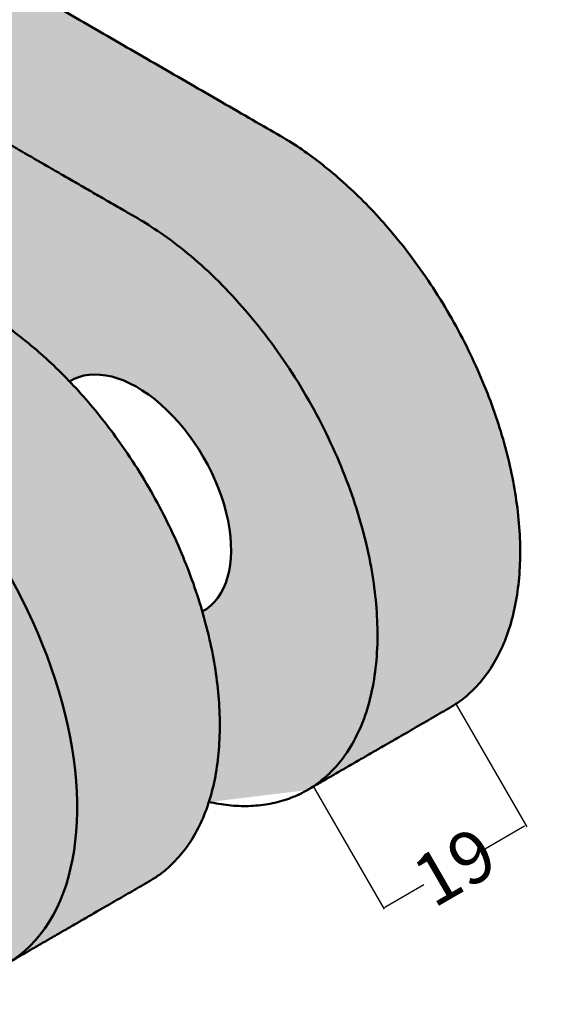
# Model space of a CAD drawing. Units: millimetres. Extents: x -24 to 183, y 0 to 191.
# Tile 1 of 1: x 120.7 to 183.4, y 6.1 to 119.6. Entities that reach past the tile are written whole.
import ezdxf

# ---------------------------------------------------------------- set-up
doc = ezdxf.new("R2010")
doc.units = ezdxf.units.MM
doc.header["$MEASUREMENT"] = 0
for name, color, linetype, lineweight in [('M-DIMS', 2, 'Continuous', 25), ('M-HATC', 7, 'Continuous', 18), ('M-OUTL', 7, 'Continuous', 50)]:
    doc.layers.add(name, color=color, linetype=linetype, lineweight=lineweight)
doc.styles.get("Standard").update_dxf_attribs({"font": 'arial.ttf'})
doc.dimstyles.get("Standard").update_dxf_attribs({"dimtxt": 6, "dimasz": 0.18, "dimexe": 0.18, "dimexo": 0.0625, "dimgap": 0.09, "dimtad": 0, "dimtoh": 1, "dimdec": 0, "dimzin": 0, "dimdsep": 46, "dimtxsty": 'Standard', "dimcen": 0.09, "dimadec": 0, "dimazin": 0, "dimtfac": 1, "dimtdec": 0, "dimtofl": 0, "dimtmove": 0, "dimatfit": 3, "dimfxl": 1, "dimtolj": 1, "dimtzin": 0, "dimarcsym": 0})

# ---------------------------------------------------------------- blocks, each defined once
blk = doc.blocks.new('*D10')
at = {"layer": 'Defpoints', "color": 0, "transparency": 16777216}
for p in [(171.0477061015821, 40.70913944972441), (154.5932234296778, 31.20913944972442), (179.1326412495718, 26.70562099750689)]:
    blk.add_point(p, dxfattribs=at)
at = {"layer": 'M-DIMS', "color": 0, "lineweight": -2, "transparency": 16777216}
for p, q in [((171.0789561015821, 40.65501286198788), (179.2226412495718, 26.54973642482568)), ((154.6244734296777, 31.15501286198789), (162.7681585776674, 17.04973642482568)), ((178.9767566768906, 26.61562099750689), (174.4657567670197, 24.01119398522857)), ((162.8340431503486, 17.29562099750689), (167.3450430602194, 19.90004800978519))]:
    blk.add_line(p, q, dxfattribs=at)
at = {"layer": 'M-DIMS', "color": 0, "transparency": 16777216}
for points in [[(178.9617566768906, 26.64160175962042), (178.9917566768906, 26.58964023539335), (179.1326412495718, 26.70562099750689)], [(162.8190431503487, 17.32160175962043), (162.8490431503486, 17.26964023539335), (162.6781585776674, 17.20562099750689)]]:
    blk.add_solid(points, dxfattribs=at)
at = {"layer": 'M-DIMS', "color": 0, "transparency": 16777216, "insert": (170.9053999136196, 21.95562099750688), "char_height": 6, "attachment_point": 5, "rotation": 29.999999999999993}
blk.add_mtext('\\A1;19', dxfattribs=at)

msp = doc.modelspace()

# ---------------------------------------------------------------- hatches: boundary and pattern name
at = {"layer": 'M-HATC'}
h = msp.add_hatch(color=256, dxfattribs=at)
h.set_gradient(color1=(244, 238, 81), color2=(244, 238, 81), tint=1)
h.paths.add_polyline_path([(64.14245464474502, 175.211638219327), (-0.8094506390879131, 137.7116382193271), (53.75014979933173, 106.2116382193271), (118.7020550831646, 143.7116382193271)])
edge = h.paths.add_edge_path()
edge.add_line((95.31936918098478, 130.2116382193271), (77.13283570151161, 119.7116382193271))
edge.add_spline(control_points=[(77.13283570151158, 119.7116382193271), (89.17924906810929, 107.2566382193724), (101.2256624347508, 94.80163821937239)], knot_values=[5.356194490192345, 5.356194490192345, 5.356194490192345, 6.356194490188707, 6.356194490192345, 6.356194490192345], weights=[1, 1, 1], degree=2, periodic=0)
edge.add_spline(control_points=[(101.2256624347947, 94.80163821932707), (110.3189291745312, 100.051638219327), (119.4121959142679, 105.301638219327)], knot_values=[6.356194490188707, 6.356194490192345, 6.356194490192345, 7.356194490192345, 7.356194490192345, 7.356194490192345], weights=[1, 1, 1], degree=2, periodic=0)
edge.add_line((119.4121959142679, 105.3016382193271), (95.31936918098478, 130.2116382193271))
edge = h.paths.add_edge_path()
edge.add_spline(control_points=[(150.7449950231889, 106.2116382193271), (134.7235250531767, 115.4616382193271), (118.7020550831646, 124.7116382193271)], knot_values=[3.356194490192345, 3.356194490192345, 3.356194490192345, 4.178416712414569, 4.178416712414569, 4.178416712414569], weights=[1, 1, 1], degree=2, periodic=0)
edge.add_spline(control_points=[(118.7020550831646, 124.7116382193271), (115.2379534680269, 126.7116382193271), (111.7738518528891, 128.7116382193271)], knot_values=[4.178416712414569, 4.178416712414569, 4.178416712414569, 4.356194490192345, 4.356194490192345, 4.356194490192345], weights=[1, 1, 1], degree=2, periodic=0)
edge.add_spline(control_points=[(111.7738518528891, 128.7116382193271), (106.960071285434, 125.9324007128871), (102.1462907179789, 123.1531632064471)], knot_values=[4.356194490192345, 4.356194490192345, 4.356194490192345, 5.356194490192345, 5.356194490192345, 5.356194490192345], weights=[1, 1, 1], degree=2, periodic=0)
edge.add_line((102.1462907179789, 123.1531632064471), (119.4121959142679, 105.301638219327))
edge.add_spline(control_points=[(119.4121959142679, 105.301638219327), (126.8513541327762, 101.006638219327), (134.2905123512845, 96.71163821932709)], knot_values=[7.356194490192345, 7.356194490192345, 7.356194490192345, 8.356194490192346, 8.356194490192346, 8.356194490192346], weights=[1, 1, 1], degree=2, periodic=0)
edge.add_spline(control_points=[(134.2905123512845, 96.71163821932709), (158.0953395036126, 82.96791485491796), (161.6862132372617, 53.72180942535438), (165.2770869709107, 24.47570399579081), (142.5556009483879, 29.39608484008592)], knot_values=[8.356194490192346, 8.356194490192346, 8.356194490192346, 9.775566349411587, 9.775566349411587, 11.19493820863083, 11.19493820863083, 11.19493820863083], weights=[1, 0.7585665602715825, 1, 0.7585665602715825, 1], degree=2, periodic=0)
edge.add_spline(control_points=[(153.8864302935499, 30.77051272237281), (162.1136716295021, 35.52051272237281), (170.3409129654543, 40.2705127223728)], knot_values=[0, 0, 0, 1, 1, 1], weights=[1, 1, 1], degree=2, periodic=0)
edge.add_spline(control_points=[(170.3409129654543, 40.2705127223728), (183.4344867248955, 47.83009105704043), (176.3482956693094, 71.67543553482938), (169.2621046137232, 95.5207800126183), (150.7449950231889, 106.2116382193271)], knot_values=[1, 1, 1, 2.178097245096171, 2.178097245096171, 3.356194490192345, 3.356194490192345, 3.356194490192345], weights=[1, 0.831469612302545, 1, 0.831469612302545, 1], degree=2, periodic=0)
edge = h.paths.add_edge_path(flags=17)
edge.add_spline(control_points=[(134.2905123512845, 96.71163821932709), (126.8513541327762, 101.006638219327), (119.4121959142679, 105.301638219327)], knot_values=[7.356194490192345, 7.356194490192345, 7.356194490192345, 8.356194490192346, 8.356194490192346, 8.356194490192346], weights=[1, 1, 1], degree=2, periodic=0)
edge.add_line((119.4121959142679, 105.301638219327), (119.4121959142679, 84.07281383496964))
edge.add_spline(control_points=[(119.4121959142679, 84.07281383496964), (123.0724490086632, 81.4513939238958), (126.4903518736498, 77.88262675949477)], knot_values=[2.966768687208849, 2.966768687208849, 2.966768687208849, 3.231438789490306, 3.231438789490306, 3.231438789490306], weights=[0.9680864183363699, 0.938243390584542, 0.9254123758008628], degree=2, periodic=0)
edge.add_ellipse((134.2905123512845, 64.71163821932709), major_axis=(7.654655446197426, -13.25825214724777), ratio=0.5773502691896262, start_angle=359.3650130620468, end_angle=540.634986937953, ccw=False)
edge.add_spline(control_points=[(141.7968427812057, 51.37100682201758), (145.5119247027769, 38.61436904653682), (142.5556009483879, 29.39608484008592)], knot_values=[1.485548755374229, 1.485548755374229, 1.485548755374229, 2.169061485720957, 2.169061485720957, 2.169061485720957], weights=[0.9974346422091759, 0.9011559533067647, 0.9183363162707197], degree=2, periodic=0)
edge.add_spline(control_points=[(142.5556009483879, 29.39608484008592), (165.2770869709107, 24.47570399579081), (161.6862132372617, 53.72180942535438), (158.0953395036126, 82.96791485491796), (134.2905123512845, 96.71163821932709)], knot_values=[8.356194490192342, 8.356194490192342, 8.356194490192342, 9.775566349411587, 9.775566349411587, 11.19493820863083, 11.19493820863083, 11.19493820863083], weights=[1, 0.7585665602715825, 1, 0.7585665602715825, 1], degree=2, periodic=0)
edge = h.paths.add_edge_path()
edge.add_spline(control_points=[(119.4121959142679, 105.301638219327), (110.3189291745312, 100.051638219327), (101.2256624347947, 94.80163821932707)], knot_values=[6.356194490188707, 6.356194490188707, 6.356194490188707, 7.356194490188707, 7.356194490188707, 7.356194490192345], weights=[1, 1, 1], degree=2, periodic=0)
edge.add_spline(control_points=[(101.2256624347947, 94.80163821932709), (108.664820653303, 90.5066382193271), (116.1039788718113, 86.21163821932711)], knot_values=[3.356194490192346, 3.356194490192346, 3.356194490192346, 3.737972267970123, 3.737972267970123, 3.737972267970123], weights=[1, 1, 1], degree=2, periodic=0)
edge.add_spline(control_points=[(116.1039788718113, 86.21163821932711), (117.7640226821475, 85.25321147856292), (119.4121959142679, 84.07281383496964)], knot_values=[3.231438789490306, 3.231438789490306, 3.231438789490306, 3.356194490192346, 3.356194490192346, 3.356194490192346], weights=[1, 0.9821533182474542, 0.9680864183363699], degree=2, periodic=0)
edge.add_line((119.4121959142679, 84.07281383496965), (119.4121959142679, 105.301638219327))
h.paths.add_polyline_path([(-0.8094506390879131, 137.7116382193271), (-0.8094506390879131, 117.7116382193271), (32.09951470472076, 98.71163821932709), (32.09951470472076, 63.71163821932707), (-0.8094506390879131, 82.71163821932709), (-0.8094506390879062, 62.71163821932709), (53.75014979933173, 31.21163821932709), (53.75014979933173, 106.2116382193271)])
h.paths.add_polyline_path([(32.09951470472076, 98.71163821932709), (29.50143849336745, 100.2116382193271), (-0.8094506390879203, 82.71163821932709), (32.09951470472076, 63.71163821932708)])
edge = h.paths.add_edge_path()
edge.add_spline(control_points=[(99.64949619990696, 57.21163821932711), (99.64949619990696, 66.96163821932711), (99.64949619990696, 76.71163821932711)], knot_values=[5.141592653589794, 5.141592653589794, 5.141592653589794, 5.446280153589794, 5.446280153589794, 5.446280153589794], weights=[1, 1, 1], degree=2, periodic=0)
edge.add_line((99.64949619990699, 76.7116382193271), (60.67835302960723, 99.2116382193271))
edge.add_spline(control_points=[(60.67835302960723, 99.2116382193271), (60.67835302960723, 67.2116382193271), (60.67835302960723, 35.2116382193271)], knot_values=[0, 0, 0, 1, 1, 1], weights=[1, 1, 1], degree=2, periodic=0)
edge.add_spline(control_points=[(60.67835302960723, 35.2116382193271), (80.16392461475712, 23.9616382193271), (99.64949619990699, 12.71163821932711)], knot_values=[1, 1, 1, 2, 2, 2], weights=[1, 1, 1], degree=2, periodic=0)
edge.add_spline(control_points=[(99.64949619990699, 12.7116382193271), (99.64949619990699, 22.4616382193271), (99.64949619990699, 32.2116382193271)], knot_values=[5.836905153589794, 5.836905153589794, 5.836905153589794, 6.141592653589794, 6.141592653589794, 6.141592653589794], weights=[1, 1, 1], degree=2, periodic=0)
edge.add_ellipse((99.64949619990699, 44.7116382193271), major_axis=(7.654655446197426, -13.25825214724777), ratio=0.5773502691896261, start_angle=150, end_angle=330, ccw=False)
edge = h.paths.add_edge_path(flags=17)
edge.add_spline(control_points=[(77.13283570151158, 119.7116382193271), (77.13283570151158, 114.2116382193271), (77.13283570151158, 108.711638219327)], knot_values=[4.356194490192345, 4.356194490192345, 4.356194490192345, 5.356194490192345, 5.356194490192345, 5.356194490192345], weights=[1, 1, 1], degree=2, periodic=0)
edge.add_spline(control_points=[(77.13283570151158, 108.711638219327), (89.17924906815313, 101.7566382193271), (101.2256624347947, 94.80163821932709)], knot_values=[3.737972267970123, 3.737972267970123, 3.737972267970123, 4.356194490192345, 4.356194490192345, 4.356194490192345], weights=[1, 1, 1], degree=2, periodic=0)
edge.add_spline(control_points=[(101.2256624347508, 94.80163821937239), (89.17924906810929, 107.2566382193724), (77.13283570151158, 119.7116382193271)], knot_values=[5.356194490192345, 5.356194490192345, 5.356194490195983, 6.356194490192345, 6.356194490192345, 6.356194490192345], weights=[1, 1, 1], degree=2, periodic=0)
edge = h.paths.add_edge_path()
edge.add_spline(control_points=[(119.2454141421726, 10.77051272237291), (121.8252656817894, 12.25999070323999), (123.649496199907, 14.85523175877608), (131.649496199907, 26.23642960525908), (123.649496199907, 46.8552317587761), (115.649496199907, 67.4740339122931), (99.64949619990696, 76.71163821932711)], knot_values=[2.780860556892677, 2.780860556892677, 2.780860556892677, 3.047197551196599, 3.047197551196599, 4.094395102393195, 4.094395102393195, 5.141592653589794, 5.141592653589794, 5.141592653589794], weights=[0.9491840326991366, 0.9659258262890693, 1, 0.8660254037844385, 1, 0.8660254037844385, 1], degree=2, periodic=0)
edge.add_spline(control_points=[(99.64949619990696, 76.71163821932711), (99.64949619990696, 66.96163821932711), (99.64949619990696, 57.21163821932711)], knot_values=[5.141592653589794, 5.141592653589794, 5.141592653589794, 5.446280153589794, 5.446280153589794, 5.446280153589794], weights=[1, 1, 1], degree=2, periodic=0)
edge.add_ellipse((99.64949619990699, 44.7116382193271), major_axis=(7.654655446197426, -13.25825214724777), ratio=0.5773502691896261, start_angle=330, end_angle=509.9999999999999, ccw=False)
edge.add_spline(control_points=[(99.64949619990699, 32.2116382193271), (99.64949619990699, 22.4616382193271), (99.64949619990699, 12.7116382193271)], knot_values=[5.836905153589794, 5.836905153589794, 5.836905153589794, 6.141592653589794, 6.141592653589794, 6.141592653589794], weights=[1, 1, 1], degree=2, periodic=0)
edge.add_spline(control_points=[(99.64949619990699, 12.71163821932711), (111.1285191633359, 6.084221221357497), (119.2454141421726, 10.77051272237291)], knot_values=[2, 2, 2, 2.780860556892677, 2.780860556892677, 2.780860556892677], weights=[1, 0.9000995774953693, 0.9491840326991366], degree=2, periodic=0)
edge = h.paths.add_edge_path()
edge.add_line((118.7020550831646, 143.7116382193271), (95.31936918098478, 130.2116382193271))
edge.add_line((95.31936918098478, 130.2116382193271), (102.1462907179789, 123.1531632064471))
edge.add_spline(control_points=[(102.1462907179789, 123.1531632064471), (106.960071285434, 125.9324007128871), (111.7738518528891, 128.7116382193271)], knot_values=[4.356194490192345, 4.356194490192345, 4.356194490192345, 5.356194490192345, 5.356194490192345, 5.356194490192345], weights=[1, 1, 1], degree=2, periodic=0)
edge.add_spline(control_points=[(111.7738518528891, 128.7116382193271), (115.2379534680269, 126.7116382193271), (118.7020550831646, 124.7116382193271)], knot_values=[4.178416712414568, 4.178416712414568, 4.178416712414568, 4.356194490192344, 4.356194490192344, 4.356194490192344], weights=[1, 1, 1], degree=2, periodic=0)
edge.add_line((118.7020550831646, 124.7116382193271), (118.7020550831646, 143.7116382193271))
h = msp.add_hatch(color=256, dxfattribs=at)
h.set_gradient(color1=(244, 238, 81), color2=(244, 238, 81), tint=1)
edge = h.paths.add_edge_path()
edge.add_spline(control_points=[(77.13283570151158, 108.711638219327), (77.13283570151158, 114.2116382193271), (77.13283570151158, 119.7116382193271)], knot_values=[4.356194490192345, 4.356194490192345, 4.356194490192345, 5.356194490192345, 5.356194490192345, 5.356194490192345], weights=[1, 1, 1], degree=2, periodic=0)
edge.add_line((77.13283570151158, 119.7116382193271), (53.75014979933173, 106.2116382193271))
edge.add_line((53.75014979933173, 106.2116382193271), (53.75014979933173, 31.21163821932707))
edge.add_line((53.75014979933173, 31.21163821932707), (60.67835302960723, 35.21163821932709))
edge.add_spline(control_points=[(60.67835302960723, 35.2116382193271), (60.67835302960723, 67.2116382193271), (60.67835302960723, 99.2116382193271)], knot_values=[0, 0, 0, 1, 1, 1], weights=[1, 1, 1], degree=2, periodic=0)
edge.add_line((60.67835302960723, 99.2116382193271), (77.13283570151158, 108.7116382193271))
edge = h.paths.add_edge_path()
edge.add_spline(control_points=[(129.6626567046299, 74.29200746748931), (128.2121653973336, 76.06903189246286), (126.674769139423, 77.68917768712181)], knot_values=[2.842732393323176, 2.842732393323176, 2.842732393323176, 2.959718296587445, 2.959718296587445, 2.959718296587445], weights=[0.9171223116143046, 0.9192697655211874, 0.9247408519506481], degree=2, periodic=0)
edge.add_spline(control_points=[(126.674769139423, 77.68917768712181), (126.5826958679184, 77.78620675354577), (126.4903518736499, 77.88262675949478)], knot_values=[2.959718296587445, 2.959718296587445, 2.959718296587445, 2.966768687208849, 2.966768687208849, 2.966768687208849], weights=[0.9247408519506481, 0.925070577972116, 0.9254123758008624], degree=2, periodic=0)
edge.add_spline(control_points=[(126.4903518736499, 77.88262675949478), (125.1497541063207, 79.2823977540787), (123.7600353652503, 80.54602783327896)], knot_values=[2.966768687208849, 2.966768687208849, 2.966768687208849, 3.069712263544142, 3.069712263544142, 3.069712263544142], weights=[0.9254123758008624, 0.9304030057906388, 0.9379672558727182], degree=2, periodic=0)
edge.add_spline(control_points=[(123.7600353652503, 80.54602783327896), (122.2074968153256, 81.95770514094174), (120.6136211690738, 83.18146756875178)], knot_values=[3.069712263544142, 3.069712263544142, 3.069712263544142, 3.18671441540082, 3.18671441540082, 3.18671441540082], weights=[0.9379672558727182, 0.946564524087908, 0.9584863481523173], degree=2, periodic=0)
edge.add_spline(control_points=[(120.6136211690738, 83.18146756875178), (120.0147834077447, 83.6412494559974), (119.4121959142679, 84.07281383496966)], knot_values=[3.18671441540082, 3.18671441540082, 3.18671441540082, 3.231438789490306, 3.231438789490306, 3.231438789490306], weights=[0.9584863481523173, 0.9630434961263034, 0.9680864183363697], degree=2, periodic=0)
edge.add_spline(control_points=[(119.4121959142679, 84.07281383496966), (119.0199233503353, 84.35375372714144), (118.6264656481512, 84.62244284625048)], knot_values=[3.231438789490306, 3.231438789490306, 3.231438789490306, 3.260806039297188, 3.260806039297188, 3.260806039297188], weights=[0.9680864183363697, 0.9713977392729884, 0.9749185064116943], degree=2, periodic=0)
edge.add_spline(control_points=[(118.6264656481512, 84.62244284625048), (117.3678455130209, 85.48194447380494), (116.1039788718113, 86.21163821932711)], knot_values=[3.260806039297188, 3.260806039297188, 3.260806039297188, 3.356194490192345, 3.356194490192345, 3.356194490192345], weights=[0.9749185064116943, 0.9863543924933733, 1], degree=2, periodic=0)
edge.add_spline(control_points=[(116.1039788718113, 86.21163821932711), (111.8084928690405, 88.6916382193271), (107.5130068662697, 91.1716382193271)], knot_values=[3.356194490192345, 3.356194490192345, 3.356194490192345, 3.57663893463679, 3.57663893463679, 3.57663893463679], weights=[1, 1, 1], degree=2, periodic=0)
edge.add_spline(control_points=[(107.5130068662697, 91.1716382193271), (104.3693346505321, 92.98663821932709), (101.2256624347947, 94.80163821932709)], knot_values=[3.57663893463679, 3.57663893463679, 3.57663893463679, 3.737972267970123, 3.737972267970123, 3.737972267970123], weights=[1, 1, 1], degree=2, periodic=0)
edge.add_spline(control_points=[(101.2256624347947, 94.80163821932709), (89.18162767796578, 101.7552649283114), (77.13759292113684, 108.7088916372958)], knot_values=[3.737972267970123, 3.737972267970123, 3.737972267970123, 4.356072419879845, 4.356072419879845, 4.356072419879845], weights=[1, 1, 1], degree=2, periodic=0)
edge.add_line((77.13283570151157, 108.711638219327), (60.67835302960723, 99.2116382193271))
edge.add_line((60.67835302960723, 99.2116382193271), (99.8447195771881, 76.59892594990174))
edge.add_spline(control_points=[(99.97475492957814, 76.52164590242904), (100.1378798240307, 76.42525480692514), (100.3009708718766, 76.32666585249011)], knot_values=[5.117048971623415, 5.117048971623415, 5.117048971623415, 5.129320817599855, 5.129320817599855, 5.129320817599855], weights=[0.9968967702000623, 0.9953635526324084, 0.9938671322846566], degree=2, periodic=0)
edge.add_spline(control_points=[(100.3009708718766, 76.32666585249011), (100.6286285674363, 76.12859593973583), (100.9560124019527, 75.92173877705902)], knot_values=[5.092505444169316, 5.092505444169316, 5.092505444169316, 5.117048971623414, 5.117048971623414, 5.117048971623414], weights=[0.9938671322846566, 0.9908743116480199, 0.988028677917995], degree=2, periodic=0)
edge.add_spline(control_points=[(100.9560124019527, 75.92173877705902), (101.2862460391653, 75.71308096927459), (101.6160138777021, 75.49560053592234)], knot_values=[5.067890674546034, 5.067890674546034, 5.067890674546034, 5.092505444169316, 5.092505444169316, 5.092505444169316], weights=[0.988028677917995, 0.9851747842049658, 0.9824689331136189], degree=2, periodic=0)
edge.add_spline(control_points=[(101.6160138777021, 75.49560053592234), (102.1164304547191, 75.16557801307957), (102.6152306653907, 74.81560168592624)], knot_values=[5.030795417572638, 5.030795417572638, 5.030795417572638, 5.067890674546034, 5.067890674546034, 5.067890674546034], weights=[0.9824689331136189, 0.9783911276699186, 0.9746495487607924], degree=2, periodic=0)
edge.add_spline(control_points=[(102.6152306653907, 74.81560168592624), (103.6180936700229, 74.11195661222713), (104.6104560145192, 73.33052013900783)], knot_values=[4.957065639950063, 4.957065639950063, 4.957065639950063, 5.030795417572638, 5.030795417572638, 5.030795417572638], weights=[0.9746495487607924, 0.9672128626872858, 0.9611044304061584], degree=2, periodic=0)
edge.add_spline(control_points=[(104.6104560145192, 73.33052013900783), (105.6134251683119, 72.5407313258447), (106.6002754642349, 71.67572813658762)], knot_values=[4.883488068876007, 4.883488068876007, 4.883488068876007, 4.957065639950062, 4.957065639950062, 4.957065639950062], weights=[0.9611044304061584, 0.9550086082728485, 0.9502355615416473], degree=2, periodic=0)
edge.add_spline(control_points=[(106.6002754642349, 71.67572813658762), (108.106571986875, 70.35541511501445), (109.5597114832291, 68.87391790201954)], knot_values=[4.772588940897321, 4.772588940897321, 4.772588940897321, 4.883488068876008, 4.883488068876008, 4.883488068876008], weights=[0.9502355615416473, 0.9430414300615662, 0.9388523470348884], degree=2, periodic=0)
edge.add_spline(control_points=[(109.5597114832291, 68.87391790201954), (110.8516035735683, 67.55681480480848), (112.0878073272173, 66.12614290817397)], knot_values=[4.674819786984862, 4.674819786984862, 4.674819786984862, 4.772588940897322, 4.772588940897322, 4.772588940897322], weights=[0.9388523470348884, 0.9351592332056611, 0.9338017218698066], degree=2, periodic=0)
edge.add_spline(control_points=[(112.0878073272173, 66.12614290817397), (113.638943035053, 64.33099687458838), (115.0807423105997, 62.38251306400263)], knot_values=[4.55254402668912, 4.55254402668912, 4.55254402668912, 4.674819786984861, 4.674819786984861, 4.674819786984861], weights=[0.9338017218698066, 0.932103939654668, 0.9340593785643667], degree=2, periodic=0)
edge.add_spline(control_points=[(115.0807423105997, 62.38251306400263), (116.5292798236757, 60.42492302971401), (117.8446599635839, 58.34337763107811)], knot_values=[4.42917907937402, 4.42917907937402, 4.42917907937402, 4.55254402668912, 4.55254402668912, 4.55254402668912], weights=[0.9340593785643667, 0.9360322357969812, 0.9417236870938861], degree=2, periodic=0)
edge.add_spline(control_points=[(117.8446599635839, 58.34337763107811), (118.8713225058487, 56.71871824481724), (119.8054692643808, 55.03626807420435)], knot_values=[4.331844561881248, 4.331844561881248, 4.331844561881248, 4.42917907937402, 4.42917907937402, 4.42917907937402], weights=[0.9417236870938861, 0.9462142225164228, 0.9530196405744161], degree=2, periodic=0)
edge.add_spline(control_points=[(119.8054692643808, 55.03626807420435), (121.1922080878205, 52.53867446936446), (122.3511098193492, 49.95830163102931)], knot_values=[4.184741853008914, 4.184741853008914, 4.184741853008914, 4.331844561881248, 4.331844561881248, 4.331844561881248], weights=[0.9530196405744161, 0.9633047424799539, 0.9788771760901379], degree=2, periodic=0)
edge.add_spline(control_points=[(122.3511098193492, 49.95830163102931), (123.0447771856724, 48.41380447289763), (123.649496199907, 46.8552317587761), (123.7106124829862, 46.69771369013003), (123.7707926063305, 46.54011834809961)], knot_values=[4.085168284068898, 4.085168284068898, 4.085168284068898, 4.175515034684617, 4.175515034684617, 4.184741853008914, 4.184741853008914, 4.184741853008914], weights=[0.9788771760901379, 0.9884413696161741, 1, 0.9988195548605517, 0.9976599114367514], degree=2, periodic=0)
edge.add_spline(control_points=[(123.7707926063305, 46.54011834809961), (124.5776705294812, 44.42712496740803), (125.2107977955467, 42.31611465871429)], knot_values=[3.9634953926215, 3.9634953926215, 3.9634953926215, 4.085168284068899, 4.085168284068899, 4.085168284068899], weights=[0.9976599114367514, 0.9823678396236314, 0.9706930540319149], degree=2, periodic=0)
edge.add_spline(control_points=[(125.2107977955467, 42.31611465871429), (125.6736053367575, 40.77299443186174), (126.0393314773653, 39.24456708280777)], knot_values=[3.876368048263354, 3.876368048263354, 3.876368048263354, 3.9634953926215, 3.9634953926215, 3.9634953926215], weights=[0.9706930540319149, 0.9623329908127651, 0.9558277578449111], degree=2, periodic=0)
edge.add_spline(control_points=[(126.0393314773653, 39.24456708280777), (126.3548486882267, 37.92597078729458), (126.5961836872144, 36.62622374004979)], knot_values=[3.80214301191095, 3.80214301191095, 3.80214301191095, 3.876368048263354, 3.876368048263354, 3.876368048263354], weights=[0.9558277578449111, 0.9502858564237563, 0.9460901130582945], degree=2, periodic=0)
edge.add_spline(control_points=[(126.5961836872144, 36.62622374004979), (126.9174285486043, 34.89610974172617), (127.1046069641274, 33.21425510536911)], knot_values=[3.70435185738841, 3.70435185738841, 3.70435185738841, 3.802143011910949, 3.802143011910949, 3.802143011910949], weights=[0.9460901130582945, 0.9405622398775964, 0.9373710204515152], degree=2, periodic=0)
edge.add_spline(control_points=[(127.1046069641274, 33.21425510536911), (127.2465779563155, 31.9386028311868), (127.3104091259611, 30.69911679832556)], knot_values=[3.630620672153618, 3.630620672153618, 3.630620672153618, 3.70435185738841, 3.70435185738841, 3.70435185738841], weights=[0.9373710204515152, 0.9349649501706391, 0.9338871843993468], degree=2, periodic=0)
edge.add_spline(control_points=[(127.3104091259611, 30.69911679832556), (127.3955283033867, 29.04625610137234), (127.3411002741898, 27.47218361842691)], knot_values=[3.532563843898478, 3.532563843898478, 3.532563843898478, 3.630620672153617, 3.630620672153617, 3.630620672153617], weights=[0.9338871843993468, 0.9324538384847469, 0.9333698597606337], degree=2, periodic=0)
edge.add_spline(control_points=[(127.3411002741898, 27.47218361842691), (127.300188233985, 26.28899698356999), (127.180615341149, 25.15821918772291)], knot_values=[3.458730317071423, 3.458730317071423, 3.458730317071423, 3.532563843898478, 3.532563843898478, 3.532563843898478], weights=[0.9333698597606337, 0.9340595932820093, 0.9360813213430013], degree=2, periodic=0)
edge.add_spline(control_points=[(127.180615341149, 25.15821918772291), (127.044748511288, 23.87335277063611), (126.8083021586305, 22.66499248616322)], knot_values=[3.374446783935056, 3.374446783935056, 3.374446783935056, 3.458730317071423, 3.458730317071423, 3.458730317071423], weights=[0.9360813213430013, 0.9383891940851565, 0.9424327908815358], degree=2, periodic=0)
edge.add_spline(control_points=[(126.8083021586305, 22.66499248616322), (126.6325923480817, 21.76702660818197), (126.4021292816593, 20.91561921939569)], knot_values=[3.311341395677428, 3.311341395677428, 3.311341395677428, 3.374446783935056, 3.374446783935056, 3.374446783935056], weights=[0.9424327908815358, 0.9454603424838158, 0.9494609282808749], degree=2, periodic=0)
edge.add_spline(control_points=[(126.4021292816593, 20.91561921939569), (126.2248036377586, 20.26051918197064), (126.0155393341565, 19.63480491824097)], knot_values=[3.262421368203812, 3.262421368203812, 3.262421368203812, 3.311341395677428, 3.311341395677428, 3.311341395677428], weights=[0.9494609282808749, 0.9525622287007962, 0.9562482769267935], degree=2, periodic=0)
edge.add_spline(control_points=[(126.0155393341565, 19.63480491824097), (125.7802944825154, 18.93140707825095), (125.5053695818401, 18.26715694529732)], knot_values=[3.206973826924972, 3.206973826924972, 3.206973826924972, 3.262421368203813, 3.262421368203813, 3.262421368203813], weights=[0.9562482769267935, 0.9604261631979532, 0.9653552567738074], degree=2, periodic=0)
edge.add_spline(control_points=[(125.5053695818401, 18.26715694529732), (125.2647817315435, 17.68586906939387), (124.9944008162674, 17.13601478791239)], knot_values=[3.157982411241067, 3.157982411241067, 3.157982411241067, 3.206973826924972, 3.206973826924972, 3.206973826924972], weights=[0.9653552567738074, 0.9697104232383605, 0.9746520453803764], degree=2, periodic=0)
edge.add_spline(control_points=[(124.9944008162674, 17.13601478791239), (124.7917726002789, 16.72394431320289), (124.5727165965067, 16.33016080220038)], knot_values=[3.120938813188745, 3.120938813188745, 3.120938813188745, 3.157982411241067, 3.157982411241067, 3.157982411241067], weights=[0.9746520453803764, 0.9783885257780115, 0.9824602969029337], degree=2, periodic=0)
edge.add_spline(control_points=[(124.5727165965067, 16.33016080220038), (124.3091183628697, 15.85630646290719), (124.0221924242566, 15.40974891923198)], knot_values=[3.075952071171273, 3.075952071171273, 3.075952071171273, 3.120938813188746, 3.120938813188746, 3.120938813188746], weights=[0.9824602969029337, 0.987405165295371, 0.9928445314164283], degree=2, periodic=0)
edge.add_spline(control_points=[(124.0221924242566, 15.40974891923198), (123.8404369956832, 15.12687363048792), (123.649496199907, 14.85523175877608), (123.5683140978384, 14.73973806312165), (123.4854899919731, 14.62630190952734)], knot_values=[3.034946113864857, 3.034946113864857, 3.034946113864857, 3.063700633839531, 3.063700633839531, 3.075952071171272, 3.075952071171272, 3.075952071171272], weights=[0.9928445314164283, 0.9963212526628074, 1, 0.998432596249194, 0.9969018674291203], degree=2, periodic=0)
edge.add_spline(control_points=[(123.4854899919731, 14.62630190952734), (123.2328877991915, 14.28033715881531), (122.9652307127422, 13.95379879127234)], knot_values=[2.997811825835947, 2.997811825835947, 2.997811825835947, 3.034946113864858, 3.034946113864858, 3.034946113864858], weights=[0.9969018674291203, 0.992262205701308, 0.9879594784250201], degree=2, periodic=0)
edge.add_spline(control_points=[(122.9652307127422, 13.95379879127234), (122.6092507510389, 13.51950759758628), (122.2273513432456, 13.1204294435816)], knot_values=[2.948919902028313, 2.948919902028313, 2.948919902028313, 2.997811825835947, 2.997811825835947, 2.997811825835947], weights=[0.9879594784250201, 0.9822944010713484, 0.9772133998627793], degree=2, periodic=0)
edge.add_spline(control_points=[(122.2273513432456, 13.1204294435816), (121.9363818855874, 12.81637148574149), (121.6308038631775, 12.53322017569058)], knot_values=[2.912007262502068, 2.912007262502068, 2.912007262502068, 2.948919902028313, 2.948919902028313, 2.948919902028313], weights=[0.9772133998627793, 0.9733773232382992, 0.9698741708558454], degree=2, periodic=0)
edge.add_spline(control_points=[(121.6308038631775, 12.53322017569058), (121.2205195242283, 12.15304706261559), (120.7847527856912, 11.81133624302551)], knot_values=[2.862862349391971, 2.862862349391971, 2.862862349391971, 2.912007262502068, 2.912007262502068, 2.912007262502068], weights=[0.9698741708558454, 0.9652101283582961, 0.9611362222017703], degree=2, periodic=0)
edge.add_spline(control_points=[(120.7847527856912, 11.81133624302551), (120.4564077324761, 11.55386120576316), (120.1141041105082, 11.31863046503682)], knot_values=[2.826105434023206, 2.826105434023206, 2.826105434023206, 2.862862349391971, 2.862862349391971, 2.862862349391971], weights=[0.9611362222017703, 0.9580892288439788, 0.9553723566239481], degree=2, periodic=0)
edge.add_spline(control_points=[(120.1141041105082, 11.31863046503682), (119.7699713416554, 11.08214273621856), (119.4121959142679, 10.86845743728019)], knot_values=[2.789361644115605, 2.789361644115605, 2.789361644115605, 2.826105434023205, 2.826105434023205, 2.826105434023205], weights=[0.9553723566239481, 0.9526564545669589, 0.9502704379250916], degree=2, periodic=0)
edge.add_spline(control_points=[(119.4121959142679, 10.86680422338807), (123.4424256961962, 13.19365847288044), (127.4726554781246, 15.52051272237282)], knot_values=[0.0101359474752899, 0.0101359474752899, 0.0101359474752899, 0.5, 0.5, 0.5], weights=[1, 1, 1], degree=2, periodic=0)
edge.add_spline(control_points=[(127.4726554781246, 15.52051272237282), (131.5862761461006, 17.89551272237281), (135.6998968140767, 20.27051272237281)], knot_values=[0.5, 0.5, 0.5, 1, 1, 1], weights=[1, 1, 1], degree=2, periodic=0)
edge.add_spline(control_points=[(135.6998968140767, 20.27051272237281), (136.1539621123821, 20.53266744457909), (136.5865086976751, 20.83096823723133)], knot_values=[1, 1, 1, 1.048792481471118, 1.048792481471118, 1.048792481471118], weights=[1, 0.9930200873881364, 0.9866183397082462], degree=2, periodic=0)
edge.add_spline(control_points=[(136.5865086976751, 20.83096823723133), (136.9176670820245, 21.05934781969398), (137.2357290184705, 21.30858758031019)], knot_values=[1.048792481471118, 1.048792481471118, 1.048792481471118, 1.085724978803377, 1.085724978803377, 1.085724978803377], weights=[0.9866183397082462, 0.9817726642684901, 0.9772582444714648], degree=2, periodic=0)
edge.add_spline(control_points=[(137.2357290184705, 21.30858758031019), (137.7660086555937, 21.72412541955322), (138.2584225013502, 22.19645227598328)], knot_values=[1.085724978803377, 1.085724978803377, 1.085724978803377, 1.146550188018983, 1.146550188018983, 1.146550188018983], weights=[0.9772582444714648, 0.9698233145729854, 0.9632868744875692], degree=2, periodic=0)
edge.add_spline(control_points=[(138.2584225013502, 22.19645227598328), (138.5573675401466, 22.4832024793678), (138.8418384740707, 22.79040575169065)], knot_values=[1.146550188018983, 1.146550188018983, 1.146550188018983, 1.183078897280162, 1.183078897280162, 1.183078897280162], weights=[0.9632868744875692, 0.9593614014384435, 0.9557599803012227], degree=2, periodic=0)
edge.add_spline(control_points=[(138.8418384740707, 22.79040575169065), (139.1385886179396, 23.11086947710986), (139.4191808804897, 23.4531491801297)], knot_values=[1.183078897280162, 1.183078897280162, 1.183078897280162, 1.220893242354295, 1.220893242354295, 1.220893242354295], weights=[0.9557599803012227, 0.9520318063691403, 0.9486508959071877], degree=2, periodic=0)
edge.add_spline(control_points=[(139.4191808804897, 23.4531491801297), (139.8668572680979, 23.99924599551215), (140.2721260020161, 24.59926038119931)], knot_values=[1.220893242354295, 1.220893242354295, 1.220893242354295, 1.280671920731201, 1.280671920731201, 1.280671920731201], weights=[0.9486508959071877, 0.9433061951400592, 0.9388293321538448], degree=2, periodic=0)
edge.add_spline(control_points=[(140.2721260020161, 24.59926038119931), (140.5232608792327, 24.97107425793451), (140.7576523147468, 25.36293735961763)], knot_values=[1.280671920731201, 1.280671920731201, 1.280671920731201, 1.317431357422621, 1.317431357422621, 1.317431357422621], weights=[0.9388293321538448, 0.9360763947188564, 0.93365161576264], degree=2, periodic=0)
edge.add_spline(control_points=[(140.7576523147468, 25.36293735961763), (141.0830933170729, 25.90702004039749), (141.3755268808085, 26.48850448529568)], knot_values=[1.317431357422621, 1.317431357422621, 1.317431357422621, 1.368155388312501, 1.368155388312501, 1.368155388312501], weights=[0.93365161576264, 0.930305684112252, 0.9275845991199414], degree=2, periodic=0)
edge.add_spline(control_points=[(141.3755268808085, 26.48850448529568), (141.6466700533705, 27.02765442133951), (141.8887940808721, 27.59768818100019)], knot_values=[1.368155388312501, 1.368155388312501, 1.368155388312501, 1.414922102988684, 1.414922102988684, 1.414922102988684], weights=[0.9275845991199414, 0.9250758039155279, 0.9230981617358409], degree=2, periodic=0)
edge.add_spline(control_points=[(141.8887940808721, 27.59768818100019), (142.1766643775072, 28.2754226015726), (142.4226727061001, 28.99479987589269)], knot_values=[1.414922102988684, 1.414922102988684, 1.414922102988684, 1.470265260532734, 1.470265260532734, 1.470265260532734], weights=[0.9230981617358409, 0.9207578441943155, 0.9191613568443742], degree=2, periodic=0)
edge.add_spline(control_points=[(142.4226727061001, 28.99479987589269), (142.490760707178, 29.19390273110689), (142.5556009483879, 29.39608484008591)], knot_values=[1.470265260532734, 1.470265260532734, 1.470265260532734, 1.485548755374229, 1.485548755374229, 1.485548755374229], weights=[0.9191613568443742, 0.9187204729617025, 0.9183363162707195], degree=2, periodic=0)
edge.add_spline(control_points=[(142.5556009483879, 29.39608484008591), (142.7432960737653, 29.98134787405721), (142.9035286953098, 30.5915899432056)], knot_values=[1.485548755374229, 1.485548755374229, 1.485548755374229, 1.529718415129709, 1.529718415129709, 1.529718415129709], weights=[0.9183363162707195, 0.9172260943934935, 0.9165896714100165], degree=2, periodic=0)
edge.add_spline(control_points=[(142.9035286953098, 30.5915899432056), (143.3840015652817, 32.42145926391575), (143.6126416122373, 34.45248245982711)], knot_values=[1.529718415129709, 1.529718415129709, 1.529718415129709, 1.66179866791104, 1.66179866791104, 1.66179866791104], weights=[0.9165896714100165, 0.9146865798082515, 0.9170201297212321], degree=2, periodic=0)
edge.add_spline(control_points=[(143.6126416122373, 34.45248245982711), (143.713072375763, 35.34461493189241), (143.764143780702, 36.27047774601957)], knot_values=[1.66179866791104, 1.66179866791104, 1.66179866791104, 1.720028544551231, 1.720028544551231, 1.720028544551231], weights=[0.9170201297212321, 0.9180489157865613, 0.9199011526878917], degree=2, periodic=0)
edge.add_spline(control_points=[(143.764143780702, 36.27047774601957), (143.8286054170071, 37.43908926285298), (143.8141447210366, 38.65544637076558)], knot_values=[1.720028544551231, 1.720028544551231, 1.720028544551231, 1.793861813952505, 1.793861813952505, 1.793861813952505], weights=[0.9199011526878917, 0.9222497186478706, 0.9259221692199169], degree=2, periodic=0)
edge.add_spline(control_points=[(143.8141447210366, 38.65544637076558), (143.8028189982979, 39.60810614478695), (143.7430996364778, 40.58628027454679)], knot_values=[1.793861813952505, 1.793861813952505, 1.793861813952505, 1.852100472733457, 1.852100472733457, 1.852100472733457], weights=[0.9259221692199169, 0.9288189472915059, 0.932539424601013], degree=2, periodic=0)
edge.add_spline(control_points=[(143.7430996364778, 40.58628027454679), (143.6681967845851, 41.81315259423612), (143.517572054451, 43.07408489058984)], knot_values=[1.852100472733457, 1.852100472733457, 1.852100472733457, 1.925809061489029, 1.925809061489029, 1.925809061489029], weights=[0.932539424601013, 0.9372481719815517, 0.9432763365187515], degree=2, periodic=0)
edge.add_spline(control_points=[(143.517572054451, 43.07408489058984), (143.3419048088425, 44.54465684249924), (143.0645134371127, 46.05133158854439)], knot_values=[1.925809061489029, 1.925809061489029, 1.925809061489029, 2.012979034199378, 2.012979034199378, 2.012979034199378], weights=[0.9432763365187515, 0.9504054234687641, 0.9593798646914953], degree=2, periodic=0)
edge.add_spline(control_points=[(143.0645134371127, 46.05133158854439), (142.8323158915082, 47.31253223755684), (142.5301351100322, 48.59179692702449)], knot_values=[2.012979034199378, 2.012979034199378, 2.012979034199378, 2.08722275193102, 2.08722275193102, 2.08722275193102], weights=[0.9593798646914953, 0.9670235045851738, 0.9760057892826022], degree=2, periodic=0)
edge.add_spline(control_points=[(142.5301351100322, 48.59179692702449), (142.2034215698478, 49.97491961764523), (141.7968427812057, 51.37100682201758)], knot_values=[2.08722275193102, 2.08722275193102, 2.08722275193102, 2.169061485720957, 2.169061485720957, 2.169061485720957], weights=[0.9760057892826022, 0.9859069476383204, 0.9974346422091759], degree=2, periodic=0)
edge.add_spline(control_points=[(141.7968427812057, 51.37100682201758), (141.7525280489804, 51.52317223829919), (141.7072795179318, 51.67543553482938), (141.6624929613182, 51.82614426707313), (141.6167947871972, 51.97693808478169)], knot_values=[2.169061485720957, 2.169061485720957, 2.169061485720957, 2.178097245096171, 2.178097245096171, 2.187040870006556, 2.187040870006556, 2.187040870006556], weights=[0.9974346422091759, 0.9987074071881719, 1, 0.9987205873030927, 0.9974606001456546], degree=2, periodic=0)
edge.add_spline(control_points=[(141.6167947871972, 51.97693808478169), (140.9517794604651, 54.17134085647821), (140.0997815197228, 56.36604687055694)], knot_values=[2.187040870006556, 2.187040870006556, 2.187040870006556, 2.314683904073241, 2.314683904073241, 2.314683904073241], weights=[0.9974606001456546, 0.9794781170616754, 0.965452398201826], degree=2, periodic=0)
edge.add_spline(control_points=[(140.0997815197228, 56.36604687055694), (139.2839372106333, 58.46762285576458), (138.3081005691592, 60.53982325286182)], knot_values=[2.314683904073241, 2.314683904073241, 2.314683904073241, 2.433530685609216, 2.433530685609216, 2.433530685609216], weights=[0.965452398201826, 0.9523932324008108, 0.9427642772030161], degree=2, periodic=0)
edge.add_spline(control_points=[(138.3081005691592, 60.53982325286182), (137.0861762910274, 63.13459359325666), (135.6376199164575, 65.63298565436963)], knot_values=[2.433530685609216, 2.433530685609216, 2.433530685609216, 2.579002148155839, 2.579002148155839, 2.579002148155839], weights=[0.9427642772030161, 0.9309781928234816, 0.9243313797502773], degree=2, periodic=0)
edge.add_spline(control_points=[(135.6376199164575, 65.63298565436963), (134.4574971723731, 67.66839783902462), (133.1455600512967, 69.60716400973533)], knot_values=[2.579002148155839, 2.579002148155839, 2.579002148155839, 2.695989522507838, 2.695989522507838, 2.695989522507838], weights=[0.9243313797502773, 0.9189860481255712, 0.9169644326127578], degree=2, periodic=0)
edge.add_spline(control_points=[(133.1455600512967, 69.60716400973533), (131.4917327990659, 72.05117163579708), (129.6626567046299, 74.29200746748931)], knot_values=[2.695989522507838, 2.695989522507838, 2.695989522507838, 2.842732393323176, 2.842732393323176, 2.842732393323176], weights=[0.9169644326127578, 0.9144286233796822, 0.9171223116143046], degree=2, periodic=0)
h.paths.add_polyline_path([(76.47887617717802, 91.77949279967994), (87.15119196487902, 85.61782840677407), (93.33332020498817, 96.32558861754949), (82.66100441728715, 102.4872530104553)], flags=24)

# ---------------------------------------------------------------- linework, layer by layer
at = {"layer": 'M-OUTL'}
for centre, major_axis, ratio, start_param, end_param in [((134.2905123512845, 64.71163821932709), (7.654655446197422, -13.25825214724777), 0.5773502691896262, 6.263991230298215, 9.443972037650745), ((99.64947289407758, 44.71155), (19.59591794226542, -33.94112549695428), 0.5773502691896258, 2e-16, 2.356194490192344)]:
    msp.add_ellipse(centre, major_axis=major_axis, ratio=ratio, start_param=start_param, end_param=end_param, dxfattribs=at)
for points, weights, knots in [([(153.8864302935499, 30.77051272237281), (162.1136716295021, 35.52051272237281), (170.3409129654543, 40.2705127223728), (183.4344867248955, 47.83009105704043), (176.3482956693094, 71.67543553482938), (169.2621046137232, 95.5207800126183), (150.7449950231889, 106.2116382193271), (131.259423438039, 117.4616382193271), (111.7738518528891, 128.7116382193271), (106.960071285434, 125.9324007128871), (102.1462907179789, 123.1531632064471)], [1, 1, 1, 0.831469612302545, 1, 0.831469612302545, 1, 1, 1, 1, 1], [0, 0, 0, 1, 1, 2.178097245096171, 2.178097245096171, 3.356194490192345, 3.356194490192345, 4.356194490192345, 4.356194490192345, 5.356194490192345, 5.356194490192345, 5.356194490192345]), ([(119.2454141421724, 10.77051272237282), (127.4726554781246, 15.52051272237282), (135.6998968140767, 20.27051272237281), (148.793470573518, 27.83009105704043), (141.7072795179318, 51.67543553482938), (134.6210884623456, 75.52078001261833), (116.1039788718113, 86.21163821932711), (96.61840728666145, 97.46163821932709), (77.13283570151158, 108.711638219327), (77.13283570151158, 114.2116382193271), (77.13283570151158, 119.7116382193271), (89.17924906815313, 107.2566382193271), (101.2256624347947, 94.80163821932707), (110.3189291745312, 100.051638219327), (119.4121959142679, 105.301638219327), (126.8513541327762, 101.006638219327), (134.2905123512845, 96.71163821932709), (158.0953395036126, 82.96791485491796), (161.6862132372617, 53.72180942535438), (165.2770869709107, 24.47570399579081), (142.5556009483879, 29.39608484008592)], [1, 1, 1, 0.831469612302545, 1, 0.831469612302545, 1, 1, 1, 1, 1, 1, 1, 1, 1, 1, 1, 0.7585665602715825, 1, 0.7585665602715825, 1], [0, 0, 0, 1, 1, 2.178097245096171, 2.178097245096171, 3.356194490192345, 3.356194490192345, 4.356194490192345, 4.356194490192345, 5.356194490192345, 5.356194490192345, 6.356194490192345, 6.356194490192345, 7.356194490192345, 7.356194490192345, 8.356194490192346, 8.356194490192346, 9.775566349411587, 9.775566349411587, 11.19493820863083, 11.19493820863083, 11.19493820863083])]:
    msp.add_rational_spline(points, weights, degree=2, knots=knots, dxfattribs=at)

# ---------------------------------------------------------------- dimensions: what is measured, and where the dimension line sits
at = {"layer": 'M-DIMS'}
dim = msp.add_aligned_dim(p1=(154.5932234296778, 31.20913944972441), p2=(171.0477061015821, 40.70913944972441), distance=-16.169870295979372, dimstyle='Standard', override={"dimclrd": 0, "dimclre": 0, "dimclrt": 0}, dxfattribs=at)
dim.commit()
dim.dimension.update_dxf_attribs({"geometry": '*D10', "text_midpoint": (170.9053999136196, 21.95562099750688)})

doc.saveas('drawing.dxf')
